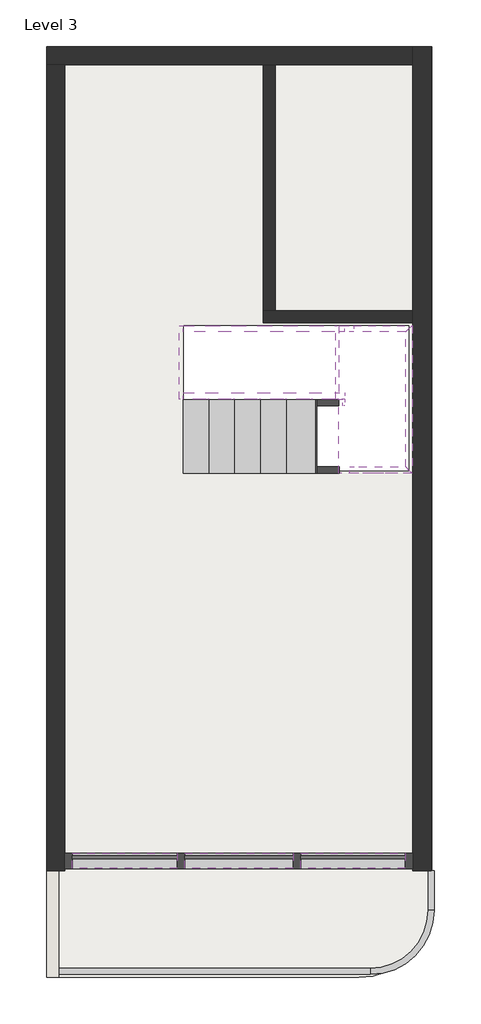
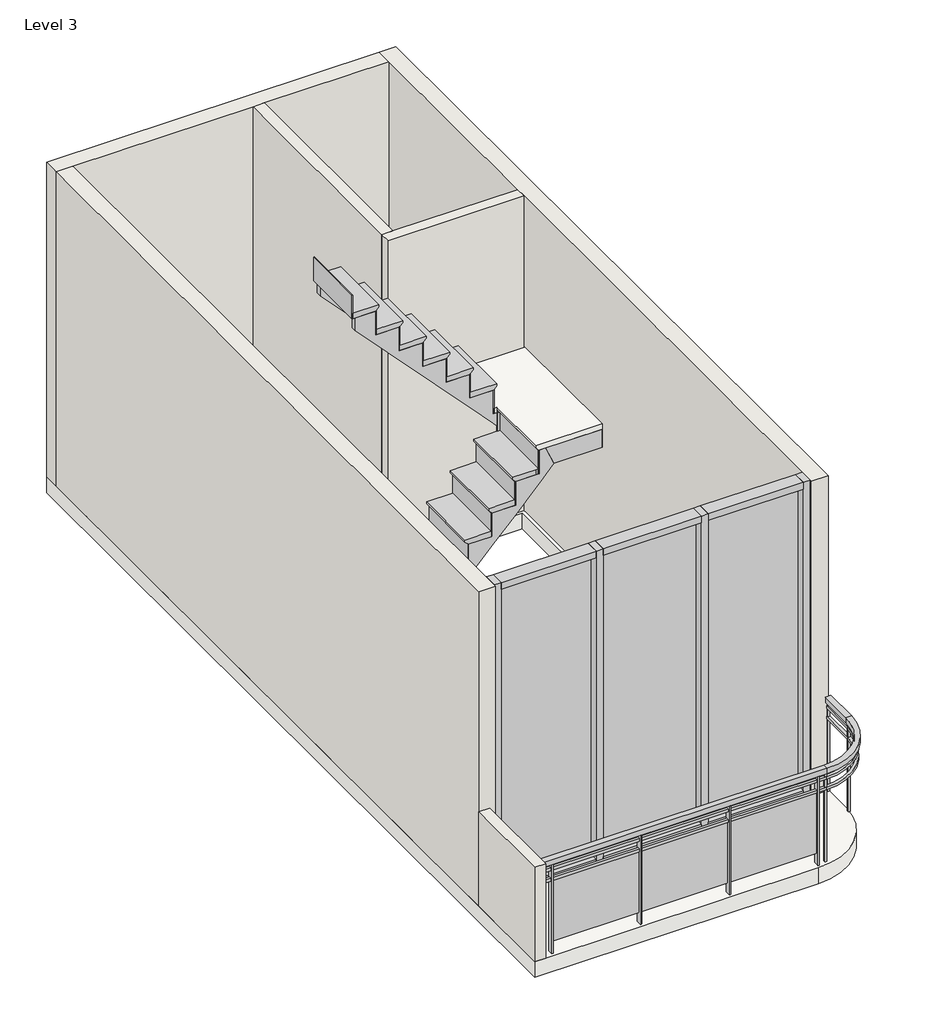
# One storey: 18 members, 6 walls, 3 plates, 2 slabs, 2 stair flights, 1 railing.
"""IFC4 building model written with IfcOpenShell, lengths in millimetres."""

from ifc_helpers import new_model, si_unit, point, frame, frame_2d, origin, place, context, project, spatial, polyline, circle_curve, trimmed, segment, composite_curve, outline, extrude, faceted_brep, transform, mapped, element, save
from ifc_brep_helpers import plane_surface, cylinder_surface, revolved_surface, advanced_brep
from components import member_024c663a, member_b7368e82, member_eaba9652, member_3f395ae9, system_panel_glazed_640eda3d, system_panel_glazed_15df7e53, non_monolithic_landing_6134172e, stair_flight_f1133b19, stair_flight_1bfa81ce

model = new_model("IFC4")

# Units and contexts
model_context = context("Model", 3, world=origin())
ifc_project = project(units=[si_unit("LENGTHUNIT", "METRE", prefix="MILLI")], contexts=[model_context])

# Site, building, storey
site = spatial("IfcSite", under=ifc_project)
building = spatial("IfcBuilding", under=site)
storey = spatial("IfcBuildingStorey", under=building, Name="Level 3", Elevation=6400.8)

# Members
placement = place(None, origin())
element("IfcMember", 1, ObjectType="Carriage - 2\" Width", at=placement, inside=storey, context=model_context, shape_type="Brep", body=[
    faceted_brep([(-3327.7134065, 4340.930501, 8178.8), (-3327.7134065, 4391.730501, 8178.8), (-3543.6134065, 4391.730501, 8178.8), (-3543.6134065, 4340.930501, 8178.8), (-3327.7134065, 4340.930501, 7950.2), (-3327.7134065, 4391.730501, 7950.2), (-3543.6134065, 4340.930501, 8407.4), (-3543.6134065, 4391.730501, 8407.4), (-3759.5134065, 4391.730501, 8407.4), (-3759.5134065, 4340.930501, 8407.4), (-3759.5134065, 4340.930501, 8636.0), (-3759.5134065, 4391.730501, 8636.0), (-3975.4134065, 4391.730501, 8636.0), (-3975.4134065, 4340.930501, 8636.0), (-3975.4134065, 4340.930501, 8864.6), (-3975.4134065, 4391.730501, 8864.6), (-4191.3134065, 4391.730501, 8864.6), (-4191.3134065, 4340.930501, 8864.6), (-4191.3134065, 4340.930501, 9093.2), (-4191.3134065, 4391.730501, 9093.2), (-4407.2134065, 4391.730501, 9093.2), (-4407.2134065, 4340.930501, 9093.2), (-4407.2134065, 4340.930501, 9321.8), (-4407.2134065, 4391.730501, 9321.8), (-4591.3634065, 4391.730501, 9321.8), (-4591.3634065, 4340.930501, 9321.8), (-3245.1634065, 4340.930501, 7772.4), (-3245.1634065, 4391.730501, 7772.4), (-3245.1634065, 4391.730501, 7950.2), (-3245.1634065, 4340.930501, 7950.2), (-3247.1348586, 4340.930501, 7772.4), (-3247.1348586, 4391.730501, 7772.4), (-4591.3634065, 4391.730501, 9195.7008155), (-4591.3634065, 4340.930501, 9195.7008155), (-3295.9634065, 4340.930501, 7824.1008155), (-3327.7134065, 4340.930501, 7857.7184625), (-3543.6134065, 4340.930501, 8086.3184625), (-3759.5134065, 4340.930501, 8314.9184625), (-3975.4134065, 4340.930501, 8543.5184625), (-4191.3134065, 4340.930501, 8772.1184625), (-4407.2134065, 4340.930501, 9000.7184625), (-3295.9634065, 4340.930501, 7950.2)], [[[0, 1, 2, 3]], [[1, 0, 4, 5]], [[6, 7, 8, 9]], [[3, 2, 7, 6]], [[10, 11, 12, 13]], [[9, 8, 11, 10]], [[14, 15, 16, 17]], [[13, 12, 15, 14]], [[18, 19, 20, 21]], [[17, 16, 19, 18]], [[22, 23, 24, 25]], [[21, 20, 23, 22]], [[26, 27, 28, 29]], [[26, 30, 31, 27]], [[32, 33, 25, 24]], [[31, 32, 24, 23, 20, 19, 16, 15, 12, 11, 8, 7, 2, 1, 5, 28, 27]], [[33, 32, 31, 30, 34, 35, 36, 37, 38, 39, 40]], [[30, 26, 29, 41, 4, 0, 3, 6, 9, 10, 13, 14, 17, 18, 21, 22, 25, 33, 40, 39, 38, 37, 36, 35, 34]], [[5, 4, 41, 29, 28]]]),
])
element("IfcMember", 2, ObjectType="Carriage - 2\" Width", at=placement, inside=storey, context=model_context, shape_type="Brep", body=[
    faceted_brep([(-4591.3634065, 4950.530501, 9195.7008155), (-4591.3634065, 4899.730501, 9195.7008155), (-4591.3634065, 4899.730501, 9321.8), (-4591.3634065, 4950.530501, 9321.8), (-3247.1348586, 4899.730501, 7772.4), (-3170.4947928, 4899.730501, 7950.2), (-3327.7134065, 4899.730501, 7950.2), (-3327.7134065, 4899.730501, 8178.8), (-3543.6134065, 4899.730501, 8178.8), (-3543.6134065, 4899.730501, 8407.4), (-3759.5134065, 4899.730501, 8407.4), (-3759.5134065, 4899.730501, 8636.0), (-3975.4134065, 4899.730501, 8636.0), (-3975.4134065, 4899.730501, 8864.6), (-4191.3134065, 4899.730501, 8864.6), (-4191.3134065, 4899.730501, 9093.2), (-4407.2134065, 4899.730501, 9093.2), (-4407.2134065, 4899.730501, 9321.8), (-4407.2134065, 4950.530501, 9000.7184625), (-4191.3134065, 4950.530501, 8772.1184625), (-3975.4134065, 4950.530501, 8543.5184625), (-3759.5134065, 4950.530501, 8314.9184625), (-3543.6134065, 4950.530501, 8086.3184625), (-3327.7134065, 4950.530501, 7857.7184625), (-3295.9634065, 4950.530501, 7824.1008155), (-3247.1348586, 4950.530501, 7772.4), (-4407.2134065, 4950.530501, 9321.8), (-4407.2134065, 4950.530501, 9093.2), (-4191.3134065, 4950.530501, 9093.2), (-4191.3134065, 4950.530501, 8864.6), (-3975.4134065, 4950.530501, 8864.6), (-3975.4134065, 4950.530501, 8636.0), (-3759.5134065, 4950.530501, 8636.0), (-3759.5134065, 4950.530501, 8407.4), (-3543.6134065, 4950.530501, 8407.4), (-3543.6134065, 4950.530501, 8178.8), (-3327.7134065, 4950.530501, 8178.8), (-3327.7134065, 4950.530501, 7950.2), (-3295.9634065, 4950.530501, 7950.2), (-3170.4947928, 4950.530501, 7950.2)], [[[0, 1, 2, 3]], [[1, 4, 5, 6, 7, 8, 9, 10, 11, 12, 13, 14, 15, 16, 17, 2]], [[1, 0, 18, 19, 20, 21, 22, 23, 24, 25, 4]], [[0, 3, 26, 27, 28, 29, 30, 31, 32, 33, 34, 35, 36, 37, 38, 39, 25, 24, 23, 22, 21, 20, 19, 18]], [[7, 36, 35, 8]], [[36, 7, 6, 37]], [[9, 34, 33, 10]], [[8, 35, 34, 9]], [[11, 32, 31, 12]], [[10, 33, 32, 11]], [[13, 30, 29, 14]], [[12, 31, 30, 13]], [[15, 28, 27, 16]], [[14, 29, 28, 15]], [[17, 26, 3, 2]], [[16, 27, 26, 17]], [[4, 25, 39, 5]], [[37, 6, 5, 39, 38]]]),
])
element("IfcMember", 3, ObjectType="Carriage - 2\" Width", at=placement, inside=storey, context=model_context, shape_type="Brep", body=[
    faceted_brep([(-4559.6134065, 4334.3702159, 6400.8), (-4424.2919545, 4334.3702159, 6400.8), (-4424.2919545, 4283.5702159, 6400.8), (-4559.6134065, 4283.5702159, 6400.8), (-3295.9634065, 4334.3702159, 7595.5008155), (-3295.9634065, 4283.5702159, 7595.5008155), (-4343.7134065, 4334.3702159, 6486.1184625), (-4127.8134065, 4334.3702159, 6714.7184625), (-3911.9134065, 4334.3702159, 6943.3184625), (-3696.0134065, 4334.3702159, 7171.9184625), (-3480.1134065, 4334.3702159, 7400.5184625), (-3295.9634065, 4334.3702159, 7721.6), (-4559.6134065, 4334.3702159, 6578.6), (-4343.7134065, 4334.3702159, 6578.6), (-4343.7134065, 4334.3702159, 6807.2), (-4127.8134065, 4334.3702159, 6807.2), (-4127.8134065, 4334.3702159, 7035.8), (-3911.9134065, 4334.3702159, 7035.8), (-3911.9134065, 4334.3702159, 7264.4), (-3696.0134065, 4334.3702159, 7264.4), (-3696.0134065, 4334.3702159, 7493.0), (-3480.1134065, 4334.3702159, 7493.0), (-3480.1134065, 4334.3702159, 7721.6), (-3480.1134065, 4283.5702159, 7721.6), (-3295.9634065, 4283.5702159, 7721.6), (-3480.1134065, 4283.5702159, 7493.0), (-3696.0134065, 4283.5702159, 7493.0), (-3696.0134065, 4283.5702159, 7264.4), (-3911.9134065, 4283.5702159, 7264.4), (-3911.9134065, 4283.5702159, 7035.8), (-4127.8134065, 4283.5702159, 7035.8), (-4127.8134065, 4283.5702159, 6807.2), (-4343.7134065, 4283.5702159, 6807.2), (-4343.7134065, 4283.5702159, 6578.6), (-4559.6134065, 4283.5702159, 6578.6)], [[[0, 1, 2, 3]], [[4, 5, 2, 1, 6, 7, 8, 9, 10]], [[11, 4, 10, 9, 8, 7, 6, 1, 0, 12, 13, 14, 15, 16, 17, 18, 19, 20, 21, 22]], [[22, 23, 24, 11]], [[2, 5, 24, 23, 25, 26, 27, 28, 29, 30, 31, 32, 33, 34, 3]], [[34, 12, 0, 3]], [[12, 34, 33, 13]], [[13, 33, 32, 14]], [[14, 32, 31, 15]], [[15, 31, 30, 16]], [[16, 30, 29, 17]], [[17, 29, 28, 18]], [[18, 28, 27, 19]], [[19, 27, 26, 20]], [[20, 26, 25, 21]], [[21, 25, 23, 22]], [[5, 4, 11, 24]]]),
])
element("IfcMember", 4, ObjectType="Carriage - 2\" Width", at=placement, inside=storey, context=model_context, shape_type="Brep", body=[
    faceted_brep([(-4559.6134065, 3775.5702159, 6400.8), (-4424.2919545, 3775.5702159, 6400.8), (-4424.2919545, 3724.7702159, 6400.8), (-4559.6134065, 3724.7702159, 6400.8), (-3128.8919545, 3775.5702159, 7772.4), (-3128.8919545, 3724.7702159, 7772.4), (-3264.2134065, 3724.7702159, 7629.1184625), (-3295.9634065, 3724.7702159, 7595.5008155), (-3480.1134065, 3724.7702159, 7400.5184625), (-3696.0134065, 3724.7702159, 7171.9184625), (-3911.9134065, 3724.7702159, 6943.3184625), (-4127.8134065, 3724.7702159, 6714.7184625), (-4343.7134065, 3724.7702159, 6486.1184625), (-3205.5320203, 3775.5702159, 7950.2), (-4559.6134065, 3775.5702159, 6578.6), (-4343.7134065, 3775.5702159, 6578.6), (-4343.7134065, 3775.5702159, 6807.2), (-4127.8134065, 3775.5702159, 6807.2), (-4127.8134065, 3775.5702159, 7035.8), (-3911.9134065, 3775.5702159, 7035.8), (-3911.9134065, 3775.5702159, 7264.4), (-3696.0134065, 3775.5702159, 7264.4), (-3696.0134065, 3775.5702159, 7493.0), (-3480.1134065, 3775.5702159, 7493.0), (-3480.1134065, 3775.5702159, 7721.6), (-3264.2134065, 3775.5702159, 7721.6), (-3264.2134065, 3775.5702159, 7950.2), (-3480.1134065, 3724.7702159, 7721.6), (-3295.9634065, 3724.7702159, 7721.6), (-3264.2134065, 3724.7702159, 7721.6), (-3205.5320203, 3724.7702159, 7950.2), (-3264.2134065, 3724.7702159, 7950.2), (-3480.1134065, 3724.7702159, 7493.0), (-3696.0134065, 3724.7702159, 7493.0), (-3696.0134065, 3724.7702159, 7264.4), (-3911.9134065, 3724.7702159, 7264.4), (-3911.9134065, 3724.7702159, 7035.8), (-4127.8134065, 3724.7702159, 7035.8), (-4127.8134065, 3724.7702159, 6807.2), (-4343.7134065, 3724.7702159, 6807.2), (-4343.7134065, 3724.7702159, 6578.6), (-4559.6134065, 3724.7702159, 6578.6)], [[[0, 1, 2, 3]], [[4, 5, 6, 7, 8, 9, 10, 11, 12, 2, 1]], [[13, 4, 1, 0, 14, 15, 16, 17, 18, 19, 20, 21, 22, 23, 24, 25, 26]], [[24, 27, 28, 29, 25]], [[5, 30, 31, 29, 28, 27, 32, 33, 34, 35, 36, 37, 38, 39, 40, 41, 3, 2, 12, 11, 10, 9, 8, 7, 6]], [[41, 14, 0, 3]], [[14, 41, 40, 15]], [[15, 40, 39, 16]], [[16, 39, 38, 17]], [[17, 38, 37, 18]], [[18, 37, 36, 19]], [[19, 36, 35, 20]], [[20, 35, 34, 21]], [[21, 34, 33, 22]], [[22, 33, 32, 23]], [[23, 32, 27, 24]], [[5, 4, 13, 30]], [[25, 29, 31, 26]], [[26, 31, 30, 13]]]),
])
element("IfcMember", 5, ObjectType="Carriage - 2\" Width", at=placement, inside=storey, context=model_context, shape_type="SweptSolid", body=[
    extrude(outline(polyline([(-3245.1634065, 4340.930501), (-3245.1634065, 4283.5702159), (-3264.2134065, 4283.5702159), (-3264.2134065, 4334.3702159), (-3295.9634065, 4334.3702159), (-3295.9634065, 4340.930501), (-3245.1634065, 4340.930501)])), frame((0.0, 0.0, 7772.4), z_axis=(0.0, 0.0, 1.0), x_axis=(1.0, 0.0, 0.0)), (0.0, 0.0, 1.0), 177.8),
])
element("IfcMember", 6, ObjectType="Carriage - 2\" Width", at=placement, inside=storey, context=model_context, shape_type="Brep", body=[
    faceted_brep([(-2737.1634065, 3775.5702159, 7772.4), (-3128.8919545, 3775.5702159, 7772.4), (-3205.5320203, 3775.5702159, 7950.2), (-2737.1634065, 3775.5702159, 7950.2), (-2686.3634065, 3724.7702159, 7772.4), (-3128.8919545, 3724.7702159, 7772.4), (-2686.3634065, 3724.7702159, 7950.2), (-3205.5320203, 3724.7702159, 7950.2)], [[[0, 1, 2, 3]], [[1, 0, 4, 5]], [[5, 4, 6, 7]], [[3, 2, 7, 6]], [[1, 5, 7, 2]], [[4, 0, 3, 6]]]),
])
element("IfcMember", 7, ObjectType="Carriage - 2\" Width", at=placement, inside=storey, context=model_context, shape_type="SweptSolid", body=[
    extrude(outline(polyline([(-2737.1634065, 3775.5702159), (-2737.1634065, 4899.730501), (-2686.3634065, 4950.530501), (-2686.3634065, 3724.7702159), (-2737.1634065, 3775.5702159)])), frame((0.0, 0.0, 7772.4), z_axis=(0.0, 0.0, 1.0), x_axis=(1.0, 0.0, 0.0)), (0.0, 0.0, 1.0), 177.8),
])
element("IfcMember", 8, ObjectType="Carriage - 2\" Width", at=placement, inside=storey, context=model_context, shape_type="Brep", body=[
    faceted_brep([(-3247.1348586, 4899.730501, 7772.4), (-2737.1634065, 4899.730501, 7772.4), (-2737.1634065, 4899.730501, 7950.2), (-3170.4947928, 4899.730501, 7950.2), (-3247.1348586, 4950.530501, 7772.4), (-2686.3634065, 4950.530501, 7772.4), (-3170.4947928, 4950.530501, 7950.2), (-2686.3634065, 4950.530501, 7950.2)], [[[0, 1, 2, 3]], [[1, 0, 4, 5]], [[5, 4, 6, 7]], [[3, 2, 7, 6]], [[1, 5, 7, 2]], [[4, 0, 3, 6]]]),
])
member_shape = member_024c663a(model_context)
element("IfcMember", 9, ObjectType="Rectangular Mullion : 2.5\" x 5\" rectangular", at=placement, inside=storey, context=model_context, shape_type="MappedRepresentation", body=[
    mapped(member_shape, transform((-2743.356559, 497.5715772, 9448.8), x_axis=(0.0, 0.0, 1.0), y_axis=(0.0, -1.0, 0.0), z_axis=(1.0, 0.0, 0.0))),
])
element("IfcMember", 10, ObjectType="Rectangular Mullion : 2.5\" x 5\" rectangular", at=placement, inside=storey, context=model_context, shape_type="MappedRepresentation", body=[
    mapped(member_shape, transform((-4642.006559, 497.5715772, 9448.8), x_axis=(0.0, 0.0, 1.0), y_axis=(0.0, -1.0, 0.0), z_axis=(1.0, 0.0, 0.0))),
])
element("IfcMember", 11, ObjectType="Rectangular Mullion : 2.5\" x 5\" rectangular", at=placement, inside=storey, context=model_context, shape_type="MappedRepresentation", body=[
    mapped(member_shape, transform((-5511.956559, 497.5715772, 6400.8), x_axis=(0.0, 0.0, -1.0), y_axis=(0.0, -1.0, 0.0), z_axis=(-1.0, 0.0, 0.0))),
])
element("IfcMember", 12, ObjectType="Rectangular Mullion : 2.5\" x 5\" rectangular", at=placement, inside=storey, context=model_context, shape_type="MappedRepresentation", body=[
    mapped(member_shape, transform((-3613.306559, 497.5715772, 6400.8), x_axis=(0.0, 0.0, -1.0), y_axis=(0.0, -1.0, 0.0), z_axis=(-1.0, 0.0, 0.0))),
])
member_2_shape = member_b7368e82(model_context)
element("IfcMember", 13, ObjectType="Rectangular Mullion : 2.5\" x 5\" rectangular", at=placement, inside=storey, context=model_context, shape_type="MappedRepresentation", body=[
    mapped(member_2_shape, transform((-4578.506559, 497.5715772, 6400.8), x_axis=(0.0, 0.0, -1.0), y_axis=(0.0, -1.0, 0.0), z_axis=(-1.0, 0.0, 0.0))),
])
element("IfcMember", 14, ObjectType="Rectangular Mullion : 2.5\" x 5\" rectangular", at=placement, inside=storey, context=model_context, shape_type="MappedRepresentation", body=[
    mapped(member_2_shape, transform((-3676.806559, 497.5715772, 9448.8), x_axis=(0.0, 0.0, 1.0), y_axis=(0.0, -1.0, 0.0), z_axis=(1.0, 0.0, 0.0))),
])
member_3_shape = member_eaba9652(model_context)
element("IfcMember", 15, ObjectType="Rectangular Mullion : 2.5\" x 5\" rectangular", at=placement, inside=storey, context=model_context, shape_type="MappedRepresentation", body=[
    mapped(member_3_shape, transform((-4610.256559, 497.5715772, 6400.8), x_axis=(1.0, 0.0, 0.0), y_axis=(0.0, -1.0, 0.0), z_axis=(0.0, 0.0, -1.0))),
])
element("IfcMember", 16, ObjectType="Rectangular Mullion : 2.5\" x 5\" rectangular", at=placement, inside=storey, context=model_context, shape_type="MappedRepresentation", body=[
    mapped(member_3_shape, transform((-3645.056559, 497.5715772, 6400.8), x_axis=(1.0, 0.0, 0.0), y_axis=(0.0, -1.0, 0.0), z_axis=(0.0, 0.0, -1.0))),
])
member_4_shape = member_3f395ae9(model_context)
element("IfcMember", 17, ObjectType="Rectangular Mullion : 2.5\" x 5\" rectangular", at=placement, inside=storey, context=model_context, shape_type="MappedRepresentation", body=[
    mapped(member_4_shape, transform((-2679.856559, 497.5715772, 6400.8), x_axis=(1.0, 0.0, 0.0), y_axis=(0.0, -1.0, 0.0), z_axis=(0.0, 0.0, -1.0))),
])
element("IfcMember", 18, ObjectType="Rectangular Mullion : 2.5\" x 5\" rectangular", at=placement, inside=storey, context=model_context, shape_type="MappedRepresentation", body=[
    mapped(member_4_shape, transform((-5575.456559, 497.5715772, 9448.8), x_axis=(-1.0, 0.0, 0.0), y_axis=(0.0, -1.0, 0.0), z_axis=(0.0, 0.0, 1.0))),
])

# Plates
system_panel_glazed_shape = system_panel_glazed_640eda3d(model_context)
element("IfcPlate", 19, ObjectType="System Panel : Glazed", at=placement, inside=storey, context=model_context, shape_type="MappedRepresentation", body=[
    mapped(system_panel_glazed_shape, transform((-5076.981559, 497.5715772, 6464.3), x_axis=(1.0, 0.0, 0.0), y_axis=(0.0, 1.0, 0.0), z_axis=(0.0, 0.0, 1.0))),
])
element("IfcPlate", 20, ObjectType="System Panel : Glazed", at=placement, inside=storey, context=model_context, shape_type="MappedRepresentation", body=[
    mapped(system_panel_glazed_shape, transform((-3178.331559, 497.5715772, 6464.3), x_axis=(1.0, 0.0, 0.0), y_axis=(0.0, 1.0, 0.0), z_axis=(0.0, 0.0, 1.0))),
])
system_panel_glazed_2_shape = system_panel_glazed_15df7e53(model_context)
element("IfcPlate", 21, ObjectType="System Panel : Glazed", at=placement, inside=storey, context=model_context, shape_type="MappedRepresentation", body=[
    mapped(system_panel_glazed_2_shape, transform((-4127.656559, 497.5715772, 6464.3), x_axis=(1.0, 0.0, 0.0), y_axis=(0.0, 1.0, 0.0), z_axis=(0.0, 0.0, 1.0))),
])

# Railing
element("IfcRailing", 22, ObjectType="Glass Panel - Bottom Fill", at=placement, inside=storey, context=model_context, shape_type="SolidModel", body=[
    advanced_brep(
    [(-5626.256559, -396.2019375, 7315.2), (-5626.256559, -396.2019375, 7264.4), (-5626.256559, -447.0019375, 7264.4), (-5626.256559, -447.0019375, 7315.2), (-3035.456559, -396.2019375, 7315.2), (-3035.456559, -396.2019375, 7264.4), (-3035.456559, -447.0019375, 7264.4), (-3035.456559, -447.0019375, 7315.2), (-2552.856559, 86.3980625, 7264.4), (-2552.856559, 86.3980625, 7315.2), (-2502.056559, 86.3980625, 7264.4), (-2502.056559, 86.3980625, 7315.2), (-2552.856559, 415.2966937, 7315.2), (-2502.056559, 415.2966937, 7315.2), (-2502.056559, 415.2966937, 7264.4), (-2552.856559, 415.2966937, 7264.4)],
    [
        (0, 1),
        (1, 2),
        (2, 3),
        (3, 0),
        (0, 4),
        (4, 5),
        (5, 1),
        (5, 6),
        (6, 2),
        (6, 7),
        (7, 3),
        (7, 4),
        (8, 5, circle_curve(frame((-3035.456559, 86.3980625, 7264.4), z_axis=(0.0, 0.0, -1.0), x_axis=(0.0, -1.0, 0.0)), 482.6)),
        (4, 9, circle_curve(frame((-3035.456559, 86.3980625, 7315.2), z_axis=(0.0, 0.0, 1.0), x_axis=(0.0, -1.0, 0.0)), 482.6)),
        (9, 8),
        (10, 6, circle_curve(frame((-3035.456559, 86.3980625, 7264.4), z_axis=(0.0, 0.0, -1.0), x_axis=(0.0, -1.0, 0.0)), 533.4)),
        (8, 10),
        (11, 7, circle_curve(frame((-3035.456559, 86.3980625, 7315.2), z_axis=(0.0, 0.0, -1.0), x_axis=(0.0, -1.0, 0.0)), 533.4)),
        (10, 11),
        (11, 9),
        (12, 13),
        (13, 14),
        (14, 15),
        (15, 12),
        (9, 12),
        (15, 8),
        (14, 10),
        (13, 11),
    ],
    [
        plane_surface(frame((-5626.256559, -421.6019375, 7315.2), z_axis=(-1.0, 0.0, 0.0), x_axis=(0.0, 1.0, 0.0))),
        plane_surface(frame((-5626.256559, -396.2019375, 7315.2), z_axis=(0.0, 1.0, 0.0), x_axis=(1.0, 0.0, 0.0))),
        plane_surface(frame((-5626.256559, -396.2019375, 7264.4), z_axis=(0.0, 0.0, -1.0), x_axis=(1.0, 0.0, 0.0))),
        plane_surface(frame((-5626.256559, -447.0019375, 7264.4), z_axis=(0.0, -1.0, 0.0), x_axis=(1.0, 0.0, 0.0))),
        plane_surface(frame((-5626.256559, -447.0019375, 7315.2), z_axis=(0.0, 0.0, 1.0), x_axis=(1.0, 0.0, 0.0))),
        revolved_surface(polyline([(-3035.456559, -396.20193750000004, 7315.2), (-3035.456559, -396.20193750000004, 7264.4)]), (-3035.456559, 86.3980625, 7315.2), (0.0, 0.0, 1.0)),
        plane_surface(frame((-3035.456559, 86.3980625, 7264.4), z_axis=(0.0, 0.0, -1.0), x_axis=(0.0, -1.0, 0.0))),
        cylinder_surface(frame((-3035.456559, 86.3980625, 7315.2), z_axis=(0.0, 0.0, 1.0), x_axis=(0.0, -1.0, 0.0)), 533.4),
        plane_surface(frame((-3035.456559, 86.3980625, 7315.2), z_axis=(0.0, 0.0, 1.0), x_axis=(0.0, -1.0, 0.0))),
        plane_surface(frame((-2527.456559, 415.2966937, 7315.2), z_axis=(0.0, 1.0, 0.0), x_axis=(0.0, 0.0, 1.0))),
        plane_surface(frame((-2552.856559, 86.3980625, 7315.2), z_axis=(-1.0, 0.0, 0.0), x_axis=(0.0, 1.0, 0.0))),
        plane_surface(frame((-2552.856559, 86.3980625, 7264.4), z_axis=(0.0, 0.0, -1.0), x_axis=(0.0, 1.0, 0.0))),
        plane_surface(frame((-2502.056559, 86.3980625, 7264.4), z_axis=(1.0, 0.0, 0.0), x_axis=(0.0, 1.0, 0.0))),
        plane_surface(frame((-2502.056559, 86.3980625, 7315.2), z_axis=(0.0, 0.0, 1.0), x_axis=(0.0, 1.0, 0.0))),
    ],
    [
        (0, [[1, 2, 3, 4]]),
        (1, [[-1, 5, 6, 7]]),
        (2, [[-2, -7, 8, 9]]),
        (3, [[-3, -9, 10, 11]]),
        (4, [[-4, -11, 12, -5]]),
        (5, [[13, -6, 14, 15]]),
        (6, [[16, -8, -13, 17]]),
        (7, [[18, -10, -16, 19]]),
        (8, [[-14, -12, -18, 20]]),
        (9, [[21, 22, 23, 24]]),
        (10, [[-15, 25, -24, 26]]),
        (11, [[-17, -26, -23, 27]]),
        (12, [[-19, -27, -22, 28]]),
        (13, [[-20, -28, -21, -25]]),
    ],
),
    advanced_brep(
    [(-5626.256559, -434.3019375, 7226.3), (-5626.256559, -408.9019375, 7226.3), (-5626.256559, -408.9019375, 7200.9), (-5626.256559, -434.3019375, 7200.9), (-3035.456559, -434.3019375, 7226.3), (-3035.456559, -408.9019375, 7226.3), (-3035.456559, -408.9019375, 7200.9), (-3035.456559, -434.3019375, 7200.9), (-2540.156559, 86.3980625, 7226.3), (-2514.756559, 86.3980625, 7226.3), (-2540.156559, 86.3980625, 7200.9), (-2514.756559, 86.3980625, 7200.9), (-2514.756559, 415.2966937, 7226.3), (-2514.756559, 415.2966937, 7200.9), (-2540.156559, 415.2966937, 7200.9), (-2540.156559, 415.2966937, 7226.3)],
    [
        (0, 1),
        (1, 2),
        (2, 3),
        (3, 0),
        (0, 4),
        (4, 5),
        (5, 1),
        (5, 6),
        (6, 2),
        (6, 7),
        (7, 3),
        (7, 4),
        (8, 5, circle_curve(frame((-3035.456559, 86.3980625, 7226.3), z_axis=(0.0, 0.0, -1.0), x_axis=(0.0, -1.0, 0.0)), 495.3)),
        (4, 9, circle_curve(frame((-3035.456559, 86.3980625, 7226.3), z_axis=(0.0, 0.0, 1.0), x_axis=(0.0, -1.0, 0.0)), 520.7)),
        (9, 8),
        (10, 6, circle_curve(frame((-3035.456559, 86.3980625, 7200.9), z_axis=(0.0, 0.0, -1.0), x_axis=(0.0, -1.0, 0.0)), 495.3)),
        (8, 10),
        (11, 7, circle_curve(frame((-3035.456559, 86.3980625, 7200.9), z_axis=(0.0, 0.0, -1.0), x_axis=(0.0, -1.0, 0.0)), 520.7)),
        (10, 11),
        (11, 9),
        (12, 13),
        (13, 14),
        (14, 15),
        (15, 12),
        (9, 12),
        (15, 8),
        (14, 10),
        (13, 11),
    ],
    [
        plane_surface(frame((-5626.256559, -421.6019375, 7213.6), z_axis=(-1.0, 0.0, 0.0), x_axis=(0.0, 1.0, 0.0))),
        plane_surface(frame((-5626.256559, -434.3019375, 7226.3), z_axis=(0.0, 0.0, 1.0), x_axis=(1.0, 0.0, 0.0))),
        plane_surface(frame((-5626.256559, -408.9019375, 7226.3), z_axis=(0.0, 1.0, 0.0), x_axis=(1.0, 0.0, 0.0))),
        plane_surface(frame((-5626.256559, -408.9019375, 7200.9), z_axis=(0.0, 0.0, -1.0), x_axis=(1.0, 0.0, 0.0))),
        plane_surface(frame((-5626.256559, -434.3019375, 7200.9), z_axis=(0.0, -1.0, 0.0), x_axis=(1.0, 0.0, 0.0))),
        plane_surface(frame((-3035.456559, 86.3980625, 7226.3), z_axis=(0.0, 0.0, 1.0), x_axis=(0.0, -1.0, 0.0))),
        revolved_surface(polyline([(-3035.456559, -408.90193750000003, 7226.3), (-3035.456559, -408.90193750000003, 7200.9)]), (-3035.456559, 86.3980625, 7213.6), (0.0, 0.0, 1.0)),
        plane_surface(frame((-3035.456559, 86.3980625, 7200.9), z_axis=(0.0, 0.0, -1.0), x_axis=(0.0, -1.0, 0.0))),
        cylinder_surface(frame((-3035.456559, 86.3980625, 7213.6), z_axis=(0.0, 0.0, 1.0), x_axis=(0.0, -1.0, 0.0)), 520.7),
        plane_surface(frame((-2527.456559, 415.2966937, 7213.6), z_axis=(0.0, 1.0, 0.0), x_axis=(0.0, 0.0, 1.0))),
        plane_surface(frame((-2514.756559, 86.3980625, 7226.3), z_axis=(0.0, 0.0, 1.0), x_axis=(0.0, 1.0, 0.0))),
        plane_surface(frame((-2540.156559, 86.3980625, 7226.3), z_axis=(-1.0, 0.0, 0.0), x_axis=(0.0, 1.0, 0.0))),
        plane_surface(frame((-2540.156559, 86.3980625, 7200.9), z_axis=(0.0, 0.0, -1.0), x_axis=(0.0, 1.0, 0.0))),
        plane_surface(frame((-2514.756559, 86.3980625, 7200.9), z_axis=(1.0, 0.0, 0.0), x_axis=(0.0, 1.0, 0.0))),
    ],
    [
        (0, [[1, 2, 3, 4]]),
        (1, [[-1, 5, 6, 7]]),
        (2, [[-2, -7, 8, 9]]),
        (3, [[-3, -9, 10, 11]]),
        (4, [[-4, -11, 12, -5]]),
        (5, [[13, -6, 14, 15]]),
        (6, [[16, -8, -13, 17]]),
        (7, [[18, -10, -16, 19]]),
        (8, [[-14, -12, -18, 20]]),
        (9, [[21, 22, 23, 24]]),
        (10, [[-15, 25, -24, 26]]),
        (11, [[-17, -26, -23, 27]]),
        (12, [[-19, -27, -22, 28]]),
        (13, [[-20, -28, -21, -25]]),
    ],
),
    advanced_brep(
    [(-5626.256559, -434.3019375, 7124.7), (-5626.256559, -408.9019375, 7124.7), (-5626.256559, -408.9019375, 7099.3), (-5626.256559, -434.3019375, 7099.3), (-3035.456559, -434.3019375, 7124.7), (-3035.456559, -408.9019375, 7124.7), (-3035.456559, -408.9019375, 7099.3), (-3035.456559, -434.3019375, 7099.3), (-2540.156559, 86.3980625, 7124.7), (-2514.756559, 86.3980625, 7124.7), (-2540.156559, 86.3980625, 7099.3), (-2514.756559, 86.3980625, 7099.3), (-2514.756559, 415.2966937, 7124.7), (-2514.756559, 415.2966937, 7099.3), (-2540.156559, 415.2966937, 7099.3), (-2540.156559, 415.2966937, 7124.7)],
    [
        (0, 1),
        (1, 2),
        (2, 3),
        (3, 0),
        (0, 4),
        (4, 5),
        (5, 1),
        (5, 6),
        (6, 2),
        (6, 7),
        (7, 3),
        (7, 4),
        (8, 5, circle_curve(frame((-3035.456559, 86.3980625, 7124.7), z_axis=(0.0, 0.0, -1.0), x_axis=(0.0, -1.0, 0.0)), 495.3)),
        (4, 9, circle_curve(frame((-3035.456559, 86.3980625, 7124.7), z_axis=(0.0, 0.0, 1.0), x_axis=(0.0, -1.0, 0.0)), 520.7)),
        (9, 8),
        (10, 6, circle_curve(frame((-3035.456559, 86.3980625, 7099.3), z_axis=(0.0, 0.0, -1.0), x_axis=(0.0, -1.0, 0.0)), 495.3)),
        (8, 10),
        (11, 7, circle_curve(frame((-3035.456559, 86.3980625, 7099.3), z_axis=(0.0, 0.0, -1.0), x_axis=(0.0, -1.0, 0.0)), 520.7)),
        (10, 11),
        (11, 9),
        (12, 13),
        (13, 14),
        (14, 15),
        (15, 12),
        (9, 12),
        (15, 8),
        (14, 10),
        (13, 11),
    ],
    [
        plane_surface(frame((-5626.256559, -421.6019375, 7112.0), z_axis=(-1.0, 0.0, 0.0), x_axis=(0.0, 1.0, 0.0))),
        plane_surface(frame((-5626.256559, -434.3019375, 7124.7), z_axis=(0.0, 0.0, 1.0), x_axis=(1.0, 0.0, 0.0))),
        plane_surface(frame((-5626.256559, -408.9019375, 7124.7), z_axis=(0.0, 1.0, 0.0), x_axis=(1.0, 0.0, 0.0))),
        plane_surface(frame((-5626.256559, -408.9019375, 7099.3), z_axis=(0.0, 0.0, -1.0), x_axis=(1.0, 0.0, 0.0))),
        plane_surface(frame((-5626.256559, -434.3019375, 7099.3), z_axis=(0.0, -1.0, 0.0), x_axis=(1.0, 0.0, 0.0))),
        plane_surface(frame((-3035.456559, 86.3980625, 7124.7), z_axis=(0.0, 0.0, 1.0), x_axis=(0.0, -1.0, 0.0))),
        revolved_surface(polyline([(-3035.456559, -408.90193750000003, 7124.7), (-3035.456559, -408.90193750000003, 7099.3)]), (-3035.456559, 86.3980625, 7112.0), (0.0, 0.0, 1.0)),
        plane_surface(frame((-3035.456559, 86.3980625, 7099.3), z_axis=(0.0, 0.0, -1.0), x_axis=(0.0, -1.0, 0.0))),
        cylinder_surface(frame((-3035.456559, 86.3980625, 7112.0), z_axis=(0.0, 0.0, 1.0), x_axis=(0.0, -1.0, 0.0)), 520.7),
        plane_surface(frame((-2527.456559, 415.2966937, 7112.0), z_axis=(0.0, 1.0, 0.0), x_axis=(0.0, 0.0, 1.0))),
        plane_surface(frame((-2514.756559, 86.3980625, 7124.7), z_axis=(0.0, 0.0, 1.0), x_axis=(0.0, 1.0, 0.0))),
        plane_surface(frame((-2540.156559, 86.3980625, 7124.7), z_axis=(-1.0, 0.0, 0.0), x_axis=(0.0, 1.0, 0.0))),
        plane_surface(frame((-2540.156559, 86.3980625, 7099.3), z_axis=(0.0, 0.0, -1.0), x_axis=(0.0, 1.0, 0.0))),
        plane_surface(frame((-2514.756559, 86.3980625, 7099.3), z_axis=(1.0, 0.0, 0.0), x_axis=(0.0, 1.0, 0.0))),
    ],
    [
        (0, [[1, 2, 3, 4]]),
        (1, [[-1, 5, 6, 7]]),
        (2, [[-2, -7, 8, 9]]),
        (3, [[-3, -9, 10, 11]]),
        (4, [[-4, -11, 12, -5]]),
        (5, [[13, -6, 14, 15]]),
        (6, [[16, -8, -13, 17]]),
        (7, [[18, -10, -16, 19]]),
        (8, [[-14, -12, -18, 20]]),
        (9, [[21, 22, 23, 24]]),
        (10, [[-15, 25, -24, 26]]),
        (11, [[-17, -26, -23, 27]]),
        (12, [[-19, -27, -22, 28]]),
        (13, [[-20, -28, -21, -25]]),
    ],
),
    extrude(outline(polyline([(-3118.006559, -447.0019375), (-3118.006559, -396.2019375), (-3105.306559, -396.2019375), (-3105.306559, -447.0019375), (-3118.006559, -447.0019375)])), frame((0.0, 0.0, 6400.8), z_axis=(0.0, 0.0, 1.0), x_axis=(1.0, 0.0, 0.0)), (0.0, 0.0, 1.0), 863.6),
    extrude(outline(polyline([(-3924.456559, -415.0667805), (-3111.656559, -415.0667805), (-3111.656559, -421.4167805), (-3924.456559, -421.4167805), (-3924.456559, -415.0667805)])), frame((0.0, 0.0, 6502.4), z_axis=(0.0, 0.0, 1.0), x_axis=(1.0, 0.0, 0.0)), (0.0, 0.0, 1.0), 596.9),
    extrude(outline(polyline([(-3930.806559, -447.0019375), (-3930.806559, -396.2019375), (-3918.106559, -396.2019375), (-3918.106559, -447.0019375), (-3930.806559, -447.0019375)])), frame((0.0, 0.0, 6400.8), z_axis=(0.0, 0.0, 1.0), x_axis=(1.0, 0.0, 0.0)), (0.0, 0.0, 1.0), 863.6),
    extrude(outline(polyline([(-4737.256559, -415.0667805), (-3924.456559, -415.0667805), (-3924.456559, -421.4167805), (-4737.256559, -421.4167805), (-4737.256559, -415.0667805)])), frame((0.0, 0.0, 6502.4), z_axis=(0.0, 0.0, 1.0), x_axis=(1.0, 0.0, 0.0)), (0.0, 0.0, 1.0), 596.9),
    extrude(outline(polyline([(-4743.606559, -447.0019375), (-4743.606559, -396.2019375), (-4730.906559, -396.2019375), (-4730.906559, -447.0019375), (-4743.606559, -447.0019375)])), frame((0.0, 0.0, 6400.8), z_axis=(0.0, 0.0, 1.0), x_axis=(1.0, 0.0, 0.0)), (0.0, 0.0, 1.0), 863.6),
    extrude(outline(polyline([(-5550.056559, -415.0667805), (-4737.256559, -415.0667805), (-4737.256559, -421.4167805), (-5550.056559, -421.4167805), (-5550.056559, -415.0667805)])), frame((0.0, 0.0, 6502.4), z_axis=(0.0, 0.0, 1.0), x_axis=(1.0, 0.0, 0.0)), (0.0, 0.0, 1.0), 596.9),
    extrude(outline(polyline([(-5556.406559, -447.0019375), (-5556.406559, -396.2019375), (-5543.706559, -396.2019375), (-5543.706559, -447.0019375), (-5556.406559, -447.0019375)])), frame((0.0, 0.0, 6400.8), z_axis=(0.0, 0.0, 1.0), x_axis=(1.0, 0.0, 0.0)), (0.0, 0.0, 1.0), 863.6),
    extrude(outline(polyline([(-2517.931559, 76.8730625), (-2536.981559, 76.8730625), (-2536.981559, 95.9230625), (-2517.931559, 95.9230625), (-2517.931559, 76.8730625)])), frame((0.0, 0.0, 6400.8), z_axis=(0.0, 0.0, 1.0), x_axis=(1.0, 0.0, 0.0)), (0.0, 0.0, 1.0), 863.6),
    extrude(outline(polyline([(-3044.981559, -431.1269375), (-3044.981559, -412.0769375), (-3025.931559, -412.0769375), (-3025.931559, -431.1269375), (-3044.981559, -431.1269375)])), frame((0.0, 0.0, 6400.8), z_axis=(0.0, 0.0, 1.0), x_axis=(1.0, 0.0, 0.0)), (0.0, 0.0, 1.0), 863.6),
    extrude(outline(polyline([(-2517.931559, 402.5966937), (-2536.981559, 402.5966937), (-2536.981559, 421.6466937), (-2517.931559, 421.6466937), (-2517.931559, 402.5966937)])), frame((0.0, 0.0, 6400.8), z_axis=(0.0, 0.0, 1.0), x_axis=(1.0, 0.0, 0.0)), (0.0, 0.0, 1.0), 863.6),
    extrude(outline(polyline([(-5632.606559, -431.1269375), (-5632.606559, -412.0769375), (-5613.556559, -412.0769375), (-5613.556559, -431.1269375), (-5632.606559, -431.1269375)])), frame((0.0, 0.0, 6400.8), z_axis=(0.0, 0.0, 1.0), x_axis=(1.0, 0.0, 0.0)), (0.0, 0.0, 1.0), 863.6),
])

# Slabs
element("IfcSlab", 23, ObjectType="6\"", at=placement, inside=storey, context=model_context, shape_type="SweptSolid", body=[
    extrude(outline(composite_curve([segment(polyline([(-2521.106559, 7274.5980625), (-2521.106559, 137.1980625)]), True, "CONTINUOUS"), segment(trimmed(circle_curve(frame_2d((-3130.706559, 137.1980625)), 609.6), [point((-2521.106559, 137.1980625))], [point((-3130.706559, -472.4019375))], False, "CARTESIAN"), True, "CONTINUOUS"), segment(polyline([(-3130.706559, -472.4019375), (-5727.856559, -472.4019375), (-5727.856559, 7274.5980625), (-2521.106559, 7274.5980625)]), True, "CONTINUOUS")], self_intersect=False), holes=[polyline([(-4584.856559, 4950.7083475), (-4584.856559, 3743.9980625), (-2711.8237097, 3743.9980625), (-2711.8237097, 4950.7083475), (-4584.856559, 4950.7083475)])]), frame((0.0, 0.0, 6248.4), z_axis=(0.0, 0.0, 1.0), x_axis=(1.0, 0.0, 0.0)), (0.0, 0.0, 1.0), 152.4),
])
non_monolithic_landing_shape = non_monolithic_landing_6134172e(model_context)
element("IfcSlab", 24, ObjectType="Non-Monolithic Landing", at=placement, inside=storey, context=model_context, shape_type="MappedRepresentation", body=[
    mapped(non_monolithic_landing_shape, transform((0.0, 0.0, 0.0), x_axis=(1.0, 0.0, 0.0), y_axis=(0.0, 1.0, 0.0), z_axis=(0.0, 0.0, 1.0))),
])

# Stair flights
stair_flight_shape = stair_flight_f1133b19(model_context)
element("IfcStairFlight", 25, ObjectType="2\" Tread 1\" Nosing 1/4\" Riser", at=placement, inside=storey, context=model_context, shape_type="MappedRepresentation", body=[
    mapped(stair_flight_shape, transform((0.0, 0.0, 0.0), x_axis=(1.0, 0.0, 0.0), y_axis=(0.0, 1.0, 0.0), z_axis=(0.0, 0.0, 1.0))),
])
stair_flight_2_shape = stair_flight_1bfa81ce(model_context)
element("IfcStairFlight", 26, ObjectType="2\" Tread 1\" Nosing 1/4\" Riser", at=placement, inside=storey, context=model_context, shape_type="MappedRepresentation", body=[
    mapped(stair_flight_2_shape, transform((0.0, 0.0, 0.0), x_axis=(1.0, 0.0, 0.0), y_axis=(0.0, 1.0, 0.0), z_axis=(0.0, 0.0, 1.0))),
])

# Walls
element("IfcWall", 27, ObjectType="4\"", at=placement, inside=storey, context=model_context, shape_type="Brep", body=[
    faceted_brep([(-2679.856559, 5076.4069788, 6400.8), (-3822.856559, 5076.4069788, 6400.8), (-3924.456559, 5076.4069788, 6400.8), (-3924.456559, 5076.4069788, 9448.8), (-3822.856559, 5076.4069788, 9448.8), (-2679.856559, 5076.4069788, 9448.8), (-2679.856559, 4974.8069788, 6400.8), (-2679.856559, 4974.8069788, 9448.8), (-3924.456559, 4974.8069788, 9448.8), (-3924.456559, 4974.8069788, 6400.8)], [[[0, 1, 2, 3, 4, 5]], [[6, 7, 8, 9]], [[2, 1, 0, 6, 9]], [[5, 4, 3, 8, 7]], [[0, 5, 7, 6]], [[3, 2, 9, 8]]]),
])
element("IfcWall", 28, ObjectType="4\"", at=placement, inside=storey, context=model_context, shape_type="SweptSolid", body=[
    extrude(outline(polyline([(-3822.856559, 7120.8966937), (-3822.856559, 5076.4069788), (-3924.456559, 5076.4069788), (-3924.456559, 7120.8966937), (-3822.856559, 7120.8966937)])), frame((0.0, 0.0, 6400.8), z_axis=(0.0, 0.0, 1.0), x_axis=(1.0, 0.0, 0.0)), (0.0, 0.0, 1.0), 3048.0),
])
element("IfcWall", 29, ObjectType="4\"", at=placement, inside=storey, context=model_context, shape_type="SweptSolid", body=[
    extrude(outline(polyline([(-5727.856559, -472.4019375), (-5727.856559, 415.2966937), (-5626.256559, 415.2966937), (-5626.256559, -472.4019375), (-5727.856559, -472.4019375)])), frame((0.0, 0.0, 6400.8), z_axis=(0.0, 0.0, 1.0), x_axis=(1.0, 0.0, 0.0)), (0.0, 0.0, 1.0), 914.4),
])
element("IfcWall", 30, ObjectType="6\"", at=placement, inside=storey, context=model_context, shape_type="Brep", body=[
    faceted_brep([(-5727.856559, 7120.8966937, 6400.8), (-5575.456559, 7120.8966937, 6400.8), (-3924.456559, 7120.8966937, 6400.8), (-3822.856559, 7120.8966937, 6400.8), (-2679.856559, 7120.8966937, 6400.8), (-2679.856559, 7120.8966937, 9448.8), (-3822.856559, 7120.8966937, 9448.8), (-3924.456559, 7120.8966937, 9448.8), (-5575.456559, 7120.8966937, 9448.8), (-5727.856559, 7120.8966937, 9448.8), (-5727.856559, 7273.2966937, 6400.8), (-5727.856559, 7273.2966937, 9448.8), (-2679.856559, 7273.2966937, 9448.8), (-2679.856559, 7273.2966937, 6400.8)], [[[0, 1, 2, 3, 4, 5, 6, 7, 8, 9]], [[10, 11, 12, 13]], [[4, 3, 2, 1, 0, 10, 13]], [[9, 8, 7, 6, 5, 12, 11]], [[0, 9, 11, 10]], [[5, 4, 13, 12]]]),
])
element("IfcWall", 31, ObjectType="6\"", at=placement, inside=storey, context=model_context, shape_type="Brep", body=[
    faceted_brep([(-2679.856559, 7273.2966937, 6400.8), (-2679.856559, 7120.8966937, 6400.8), (-2679.856559, 5076.4069788, 6400.8), (-2679.856559, 4974.8069788, 6400.8), (-2679.856559, 415.2966937, 6400.8), (-2679.856559, 415.2966937, 9448.8), (-2679.856559, 4974.8069788, 9448.8), (-2679.856559, 5076.4069788, 9448.8), (-2679.856559, 7120.8966937, 9448.8), (-2679.856559, 7273.2966937, 9448.8), (-2527.456559, 7273.2966937, 6400.8), (-2527.456559, 7273.2966937, 9448.8), (-2527.456559, 415.2966937, 9448.8), (-2527.456559, 415.2966937, 6400.8)], [[[0, 1, 2, 3, 4, 5, 6, 7, 8, 9]], [[10, 11, 12, 13]], [[4, 3, 2, 1, 0, 10, 13]], [[5, 4, 13, 12]], [[9, 8, 7, 6, 5, 12, 11]], [[0, 9, 11, 10]]]),
])
element("IfcWall", 32, ObjectType="6\"", at=placement, inside=storey, context=model_context, shape_type="Brep", body=[
    faceted_brep([(-5575.456559, 415.2966937, 6400.8), (-5575.456559, 7120.8966937, 6400.8), (-5575.456559, 7120.8966937, 9448.8), (-5575.456559, 415.2966937, 9448.8), (-5727.856559, 415.2966937, 6400.8), (-5727.856559, 415.2966937, 7315.2), (-5727.856559, 415.2966937, 9448.8), (-5727.856559, 7120.8966937, 9448.8), (-5727.856559, 7120.8966937, 6400.8), (-5626.256559, 415.2966937, 6400.8)], [[[0, 1, 2, 3]], [[4, 5, 6, 7, 8]], [[1, 0, 9, 4, 8]], [[3, 2, 7, 6]], [[0, 3, 6, 5, 4, 9]], [[2, 1, 8, 7]]]),
])

save(model, "model.ifc")

# Revit data of these elements
# Type "Rectangular Mullion : 2.5\" x 5\" rectangular"
#   built-in parameter 1007304 = 0.416667 (stored number, unit not read)
#   built-in parameter 1007301 = 0.104167 (stored number, unit not read)
#   built-in parameter 1007300 = 0.104167 (stored number, unit not read)
# Type "System Panel : Glazed"
#   Construction Type Id = "GSP4R"
#   Analytic Construction = "1/8 in Pilkington single glazing"
#   Visual Light Transmittance = 0.9
#   Solar Heat Gain Coefficient = 0.86
#   Heat Transfer Coefficient (U) = 1.18115 BTU/(h·ft²·°F)
# Type "Glass Panel - Bottom Fill"
#   Assembly Code = "C2010400"
#   built-in parameter 1008612 = 0.0416667 (stored number, unit not read)
#   built-in parameter 1008611 = 0.0416667 (stored number, unit not read)
#   built-in parameter 1008609 = 0.333333 (stored number, unit not read)
#   built-in parameter 1008604 = 0.166667 (stored number, unit not read)
#   built-in parameter 1008603 = 0.166667 (stored number, unit not read)
#   Railing Height = 3' - 0"
#   built-in parameter 1008630 = 2
#   built-in parameter 1008610 = 2
#   built-in parameter 1008618 = Baluster - Square : 3/4"
# Type "6\""
#   Assembly Code = "B1010"
#   Function = 0
#   Layers, outside or top first: 0' - 6" no material (function 1)
# Type "4\""
#   Assembly Code = "B2010"
#   Layers, outside or top first: 0' - 4" no material (function 1)
# Type "6\""
#   Assembly Code = "B2010"
#   Layers, outside or top first: 0' - 6" "ext wall" (function 1)
# Elements 1, 2, 3, 4, 5, 6, 7, 8 (IfcMember, "Carriage - 2\" Width")
#   Phase Created = New Construction
# Elements 9, 10, 11, 12, 13, 14, 15, 16, 17, 18 (IfcMember, "Rectangular Mullion : 2.5\" x 5\" rectangular")
#   Phase Created = New Construction
#   Materials on its faces: "Aluminum"
# Elements 19, 20, 21 (IfcPlate, "System Panel : Glazed")
#   Phase Created = New Construction
#   Materials on its faces: "Glass"
# Element 22 (IfcRailing, "Glass Panel - Bottom Fill")
#   Phase Created = New Construction
#   Materials on its faces: "Glass"
# Element 23 (IfcSlab, "6\"")
#   Height Offset From Level = 0' - 0"
#   Phase Created = New Construction
#   Materials on its faces: "Default Floor"
# Element 24 (IfcSlab, "Non-Monolithic Landing")
#   Phase Created = New Construction
# Elements 25, 26 (IfcStairFlight, "2\" Tread 1\" Nosing 1/4\" Riser")
#   Phase Created = New Construction
# Elements 27, 28 (IfcWall, "4\"")
#   Top Offset = 0' - 0"
#   Base Offset = 0' - 0"
#   Unconnected Height = 10' - 0"
#   wall height = 10' - 0"
#   Phase Created = New Construction
#   Base Constraint = Level 3
#   Materials on its faces: "Default Wall"
# Element 29 (IfcWall, "4\"")
#   Top Offset = 0' - 0"
#   Base Offset = 0' - 0"
#   Unconnected Height = 3' - 0"
#   wall height = 3' - 0"
#   Phase Created = New Construction
#   Base Constraint = Level 3
#   Materials on its faces: "Default Wall"
# Elements 30, 31, 32 (IfcWall, "6\"")
#   Top Offset = 0' - 0"
#   Base Offset = 0' - 0"
#   Unconnected Height = 10' - 0"
#   wall height = 10' - 0"
#   Phase Created = New Construction
#   Base Constraint = Level 3
#   Materials on its faces: "ext wall"
# Materials
#   "ext wall": class "Generic", colour RGB 187 179 160, transparency 0, Cost = 0
#   "Aluminum": class "Metal", colour RGB 247 247 247, transparency 0, Description = "Aluminum 6061", Cost = 0
#   "Glass": class "Glass", colour RGB 0 128 192, transparency 0.75, Description = "Soda Lime Glass", Cost = 0
#   "Default Floor": colour RGB 128 128 128, transparency 0
#   "Default Wall": colour RGB 128 128 128, transparency 0
